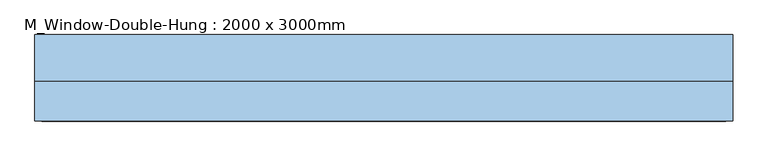
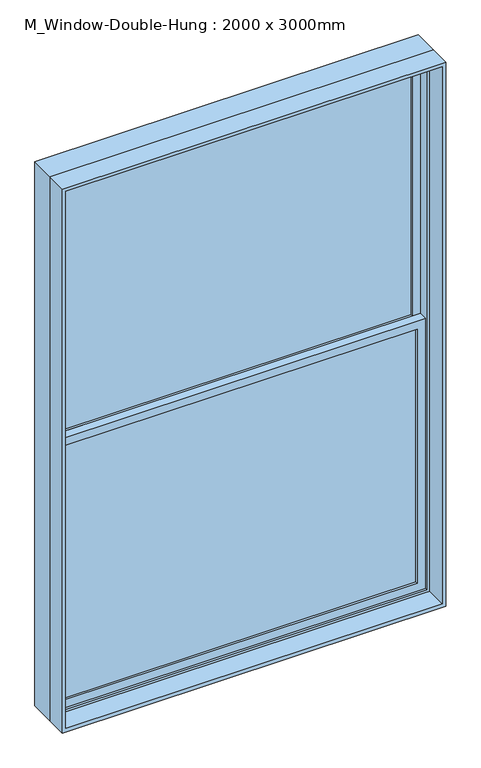
"""IFC4 building model written with IfcOpenShell, lengths in millimetres: window geometry, M_Window-Double-Hung : 2000 x 3000mm."""

from ifc_helpers import new_model, si_unit, frame, origin, place, context, project, spatial, polyline, outline, extrude, source, transform, mapped, element, save


def m_window_double_hung_2000_x_3000mm_b5dbafc5(model_context):
    return source(origin(), model_context, "Body", "SweptSolid", [
        extrude(outline(polyline([(923.8, 44.45), (923.8, 38.1), (-923.8, 38.1), (-923.8, 44.45), (923.8, 44.45)])), frame((0.0, 0.0, 990.6), z_axis=(0.0, 0.0, 1.0), x_axis=(1.0, 0.0, 0.0)), (0.0, 0.0, 1.0), 1401.575),
        extrude(outline(polyline([(-923.8, 31.75), (923.8, 31.75), (923.8, 25.4), (-923.8, 25.4), (-923.8, 31.75)])), frame((0.0, 0.0, 990.6), z_axis=(0.0, 0.0, 1.0), x_axis=(1.0, 0.0, 0.0)), (0.0, 0.0, 1.0), 1401.575),
        extrude(outline(polyline([(923.8, 88.9), (923.8, 82.55), (-923.8, 82.55), (-923.8, 88.9), (923.8, 88.9)])), frame((0.0, 0.0, 2436.625), z_axis=(0.0, 0.0, 1.0), x_axis=(1.0, 0.0, 0.0)), (0.0, 0.0, 1.0), 1401.575),
        extrude(outline(polyline([(-923.8, 76.2), (923.8, 76.2), (923.8, 69.85), (-923.8, 69.85), (-923.8, 76.2)])), frame((0.0, 0.0, 2436.625), z_axis=(0.0, 0.0, 1.0), x_axis=(1.0, 0.0, 0.0)), (0.0, 0.0, 1.0), 1401.575),
        extrude(outline(polyline([(2436.625, -968.25), (946.15, -968.25), (946.15, 968.25), (2436.625, 968.25), (2436.625, -968.25)]), holes=[polyline([(2392.175, 923.8), (990.6, 923.8), (990.6, -923.8), (2392.175, -923.8), (2392.175, 923.8)])]), frame((0.0, 12.7, 0.0), z_axis=(0.0, 1.0, 0.0), x_axis=(0.0, 0.0, 1.0)), (0.0, 0.0, 1.0), 44.45),
        extrude(outline(polyline([(3882.65, -968.25), (2392.175, -968.25), (2392.175, 968.25), (3882.65, 968.25), (3882.65, -968.25)]), holes=[polyline([(3838.2, 923.8), (2436.625, 923.8), (2436.625, -923.8), (3838.2, -923.8), (3838.2, 923.8)])]), frame((0.0, 57.15, 0.0), z_axis=(0.0, 1.0, 0.0), x_axis=(0.0, 0.0, 1.0)), (0.0, 0.0, 1.0), 44.45),
        extrude(outline(polyline([(3914.4, -1000.0), (914.4, -1000.0), (914.4, 1000.0), (3914.4, 1000.0), (3914.4, -1000.0)]), holes=[polyline([(3882.65, 968.25), (946.15, 968.25), (946.15, -968.25), (3882.65, -968.25), (3882.65, 968.25)])]), frame((0.0, 0.0, 0.0), z_axis=(0.0, 1.0, 0.0), x_axis=(0.0, 0.0, 1.0)), (0.0, 0.0, 1.0), 133.35),
        extrude(outline(polyline([(3914.4, 1000.0), (3914.4, -1000.0), (914.4, -1000.0), (914.4, 1000.0), (3914.4, 1000.0)]), holes=[polyline([(3895.35, 980.95), (933.45, 980.95), (933.45, -980.95), (3895.35, -980.95), (3895.35, 980.95)])]), frame((0.0, -114.3, 0.0), z_axis=(0.0, 1.0, 0.0), x_axis=(0.0, 0.0, 1.0)), (0.0, 0.0, 1.0), 114.3),
    ])


if __name__ == "__main__":
    model = new_model("IFC4")
    model_context = context("Model", 3, world=origin())
    ifc_project = project(units=[si_unit("LENGTHUNIT", "METRE", prefix="MILLI")], contexts=[model_context])
    site = spatial("IfcSite", under=ifc_project)
    building = spatial("IfcBuilding", under=site)
    placement = place(None, origin())
    m_window_double_hung_2000_x_3000mm_shape = m_window_double_hung_2000_x_3000mm_b5dbafc5(model_context)
    element("IfcWindow", 1, ObjectType="M_Window-Double-Hung : 2000 x 3000mm", at=placement, inside=building, context=model_context, shape_type="MappedRepresentation", body=[
        mapped(m_window_double_hung_2000_x_3000mm_shape, transform((0.0, 0.0, 0.0), x_axis=(1.0, 0.0, 0.0), y_axis=(0.0, 1.0, 0.0), z_axis=(0.0, 0.0, 1.0))),
    ])
    save(model, "model.ifc")

# Revit data of these elements
# Type "M_Window-Double-Hung : 2000 x 3000mm"
#   Type Mark = "21"
#   Fire Rating = "0.5h"
#   Construction Type Id = "DG-DR"
#   Assembly Code = "B2020100"
#   Analytic Construction = "Double glazing - domestic"
#   Wall Thickness [instance default] = 150 mm
#   Window Inset [instance default] = 0 mm
#   Visual Light Transmittance = 0.81
#   Thermal Resistance (R) = 0.319569 (m²·K)/W
#   Solar Heat Gain Coefficient = 0.76
#   Muntin Width = 1847.6 mm
#   Muntin Height = 1401.575 mm
#   Interior Wall Closure [instance default] = 35.7 mm
#   Rough Width = 2015 mm
#   Rough Height = 3015 mm
#   Frame Extension [instance default] = 31.75 mm
#   Exterior Wall Closure [instance default] = 12.7 mm
#   Extension Jamb [instance default] = 35.7 mm
#   Heat Transfer Coefficient (U) = 3.12929 W/(m²·K)
#   Height = 3000 mm
#   Width = 2000 mm
#   Define Thermal Properties by = 1
#   Top Muntin Visibility = yes
#   Indicator Visibility [instance default] = yes
#   Extension Jamb Visibility [instance default] = yes
#   Interior Trim Visibility [instance default] = yes
#   Exterior Trim Visibility [instance default] = yes
#   Define Thermal Properties by = 1
#   Bottom Muntin Visibility = yes
#   Muntin Pattern = M_Muntin Pattern_2x2 : M_Muntin Pattern_2x2
#   Interior Trim Material = Wood - Stained
#   Interior Trim = M_Trim-Window-Interior-Flat : Picture Frame
#   Exterior Trim Material = Clad - White
#   Exterior Trim = M_Trim-Window-Exterior-Flat : with Sill
#   Glass Panel Material = Glass
#   Exterior Frame Material = Clad - White
#   Interior Frame Material = Wood - Stained
#   Wall Closure = (empty or 0)
# Element 1 (IfcWindow, "M_Window-Double-Hung : 2000 x 3000mm")
#   Wall Thickness = 228.6 mm
#   Extension Jamb = 114.3 mm
#   Materials on its faces: "Wood - Stained", "Glass", "Clad - White"
# Materials
#   "Wood - Stained": class "Wood", colour RGB 224 178 126, transparency 0, Cost = 0
#   "Clad - White": class "Wood", colour RGB 242 242 238, transparency 0, Cost = 0
#   "Glass": class "Glass", colour RGB 0 128 192, transparency 0.9, Description = "Soda Lime Glass", Cost = 0
